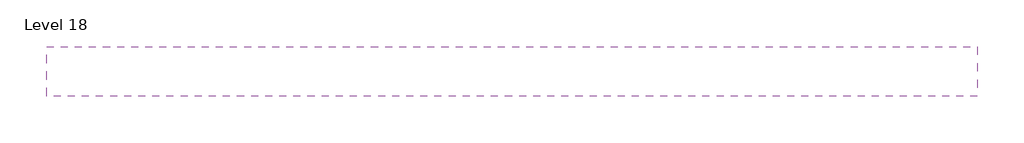
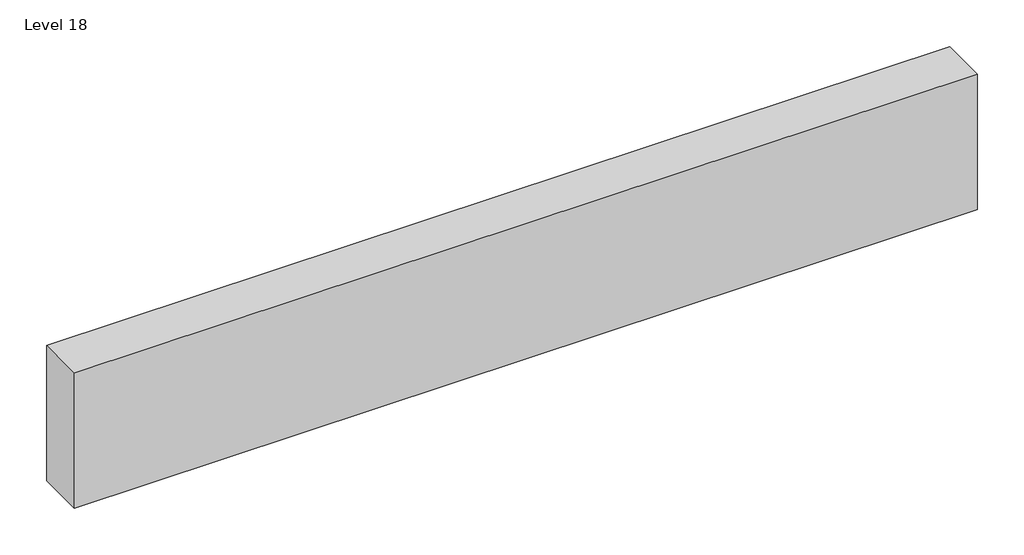
# One storey: 1 proxy.
"""IFC4 building model written with IfcOpenShell, lengths in millimetres."""

from ifc_helpers import new_model, si_unit, origin, place, context, project, spatial, transform, mapped, element, save
from components import generic_models_13_generic_models_13_3d13953a

model = new_model("IFC4")

# Units and contexts
model_context = context("Model", 3, world=origin())
ifc_project = project(units=[si_unit("LENGTHUNIT", "METRE", prefix="MILLI")], contexts=[model_context])

# Site, building, storey
site = spatial("IfcSite", under=ifc_project)
building = spatial("IfcBuilding", under=site)
storey = spatial("IfcBuildingStorey", under=building, Name="Level 18", Elevation=29260.8)

# Proxy
placement = place(None, origin())
generic_models_13_generic_models_13_shape = generic_models_13_generic_models_13_3d13953a(model_context)
element("IfcBuildingElementProxy", 1, Name="Generic Models 13 : Generic Models 13", ObjectType="Generic Models 13 : Generic Models 13", at=placement, inside=storey, context=model_context, shape_type="MappedRepresentation", body=[
    mapped(generic_models_13_generic_models_13_shape, transform((0.0, 0.0, 0.0), x_axis=(1.0, 0.0, 0.0), y_axis=(0.0, 1.0, 0.0), z_axis=(0.0, 0.0, 1.0))),
])

save(model, "model.ifc")

# Revit data of these elements
# Element 1 (IfcBuildingElementProxy, "Generic Models 13 : Generic Models 13")
#   Phase Created = New Construction
